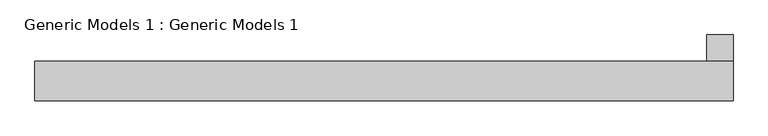
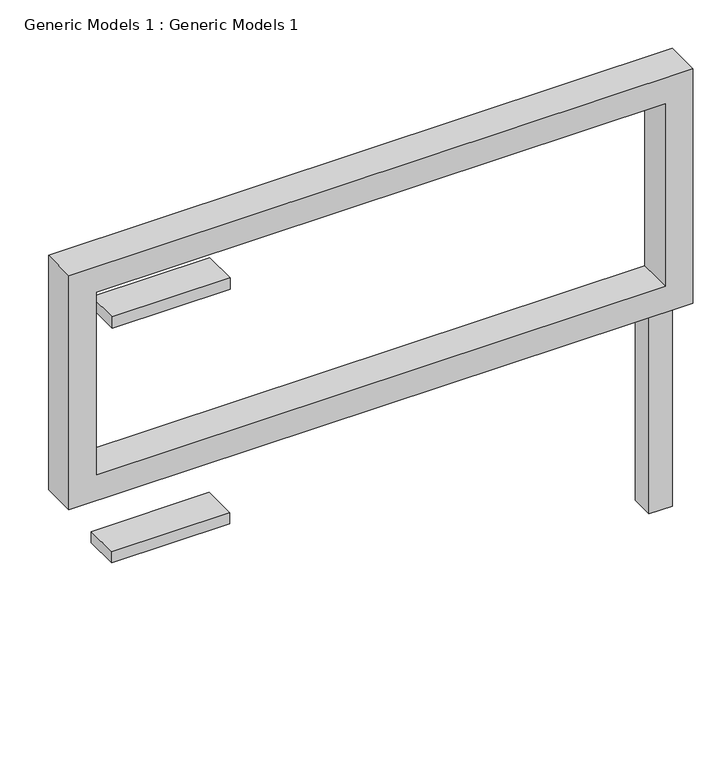
"""IFC4 building model written with IfcOpenShell, lengths in millimetres: proxy geometry, Generic Models 1 : Generic Models 1."""

from ifc_helpers import new_model, si_unit, frame, origin, origin_with_axes, place, context, project, spatial, polyline, outline, extrude, source, transform, mapped, element, save


def generic_models_1_generic_models_1_b53c1211(model_context):
    return source(origin(), model_context, "Body", "SweptSolid", [
        extrude(outline(polyline([(-10396.84011, -2343.197359), (-11920.84011, -2343.197359), (-11920.84011, -1885.997359), (-10396.84011, -1885.997359), (-10396.84011, -2343.197359)])), frame((0.0, 0.0, 2128.7275795), z_axis=(0.0, 0.0, 1.0), x_axis=(1.0, 0.0, 0.0)), (0.0, 0.0, 1.0), 152.4),
        extrude(outline(polyline([(-10392.0551496, -2343.197359), (-11916.0551496, -2343.197359), (-11916.0551496, -1885.997359), (-10392.0551496, -1885.997359), (-10392.0551496, -2343.197359)])), frame((0.0, 0.0, 5334.0), z_axis=(0.0, 0.0, 1.0), x_axis=(1.0, 0.0, 0.0)), (0.0, 0.0, 1.0), 152.4),
        extrude(outline(polyline([(-4715.1551496, -1885.997359), (-4715.1551496, -1581.197359), (-4410.3551496, -1581.197359), (-4410.3551496, -1885.997359), (-4715.1551496, -1885.997359)])), origin_with_axes(), (0.0, 0.0, 1.0), 3048.0),
        extrude(outline(polyline([(6248.4, -4410.3551496), (6248.4, -12474.9495996), (3048.0, -12474.9495996), (3048.0, -4410.3551496), (6248.4, -4410.3551496)]), holes=[polyline([(5892.8, -4765.9551496), (3403.6, -4765.9551496), (3403.6, -12119.3495996), (5892.8, -12119.3495996), (5892.8, -4765.9551496)])]), frame((0.0, -2343.197359, 0.0), z_axis=(0.0, 1.0, 0.0), x_axis=(0.0, 0.0, 1.0)), (0.0, 0.0, 1.0), 457.2),
    ])


if __name__ == "__main__":
    model = new_model("IFC4")
    model_context = context("Model", 3, world=origin())
    ifc_project = project(units=[si_unit("LENGTHUNIT", "METRE", prefix="MILLI")], contexts=[model_context])
    site = spatial("IfcSite", under=ifc_project)
    building = spatial("IfcBuilding", under=site)
    placement = place(None, origin())
    generic_models_1_generic_models_1_shape = generic_models_1_generic_models_1_b53c1211(model_context)
    element("IfcBuildingElementProxy", 1, Name="Generic Models 1 : Generic Models 1", ObjectType="Generic Models 1 : Generic Models 1", at=placement, inside=building, context=model_context, shape_type="MappedRepresentation", body=[
        mapped(generic_models_1_generic_models_1_shape, transform((0.0, 0.0, 0.0), x_axis=(1.0, 0.0, 0.0), y_axis=(0.0, 1.0, 0.0), z_axis=(0.0, 0.0, 1.0))),
    ])
    save(model, "model.ifc")

# Revit data of these elements
# Element 1 (IfcBuildingElementProxy, "Generic Models 1 : Generic Models 1")
#   Materials on its faces: "Gypsum Wall Board"
# Materials
#   "Gypsum Wall Board": class "Generic", colour RGB 127 127 127, transparency 0, Description = "Gypsum Wall Board", Cost = 0
